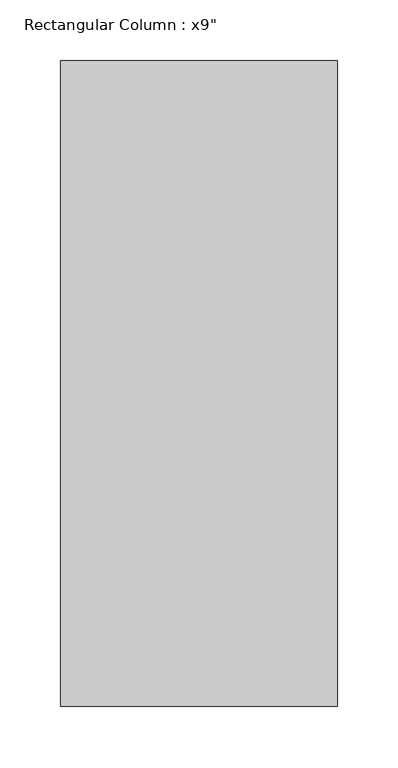
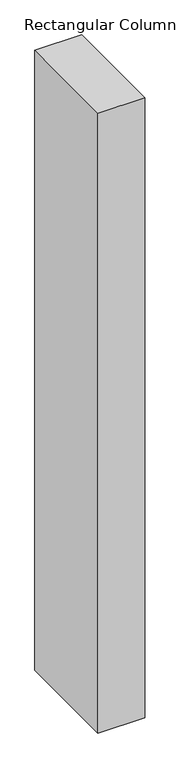
"""IFC4 building model written with IfcOpenShell, lengths in millimetres: column geometry."""

from ifc_helpers import new_model, si_unit, frame, origin, place, context, project, spatial, polyline, outline, extrude, source, transform, mapped, element, save


def column_8ec85f3f(model_context):
    return source(origin(), model_context, "Body", "SweptSolid", [
        extrude(outline(polyline([(114.3, 266.7), (114.3, -266.7), (-114.3, -266.7), (-114.3, 266.7), (114.3, 266.7)])), frame((0.0, 0.0, 6400.8), z_axis=(0.0, 0.0, 1.0), x_axis=(1.0, 0.0, 0.0)), (0.0, 0.0, 1.0), 3200.4),
    ])


if __name__ == "__main__":
    model = new_model("IFC4")
    model_context = context("Model", 3, world=origin())
    ifc_project = project(units=[si_unit("LENGTHUNIT", "METRE", prefix="MILLI")], contexts=[model_context])
    site = spatial("IfcSite", under=ifc_project)
    building = spatial("IfcBuilding", under=site)
    placement = place(None, origin())
    column_shape = column_8ec85f3f(model_context)
    element("IfcColumn", 1, ObjectType="Rectangular Column : x9\"", at=placement, inside=building, context=model_context, shape_type="MappedRepresentation", body=[
        mapped(column_shape, transform((0.0, 0.0, 0.0), x_axis=(1.0, 0.0, 0.0), y_axis=(0.0, 1.0, 0.0), z_axis=(0.0, 0.0, 1.0))),
    ])
    save(model, "model.ifc")

# Revit data of these elements
# Type "Rectangular Column : x9\""
#   Assembly Code = "B1010200"
#   Depth = 1' - 9"
#   Offset Base = 0' - 0"
#   Offset Top = 0' - 0"
#   Width = 0' - 9"
#   Material = none
